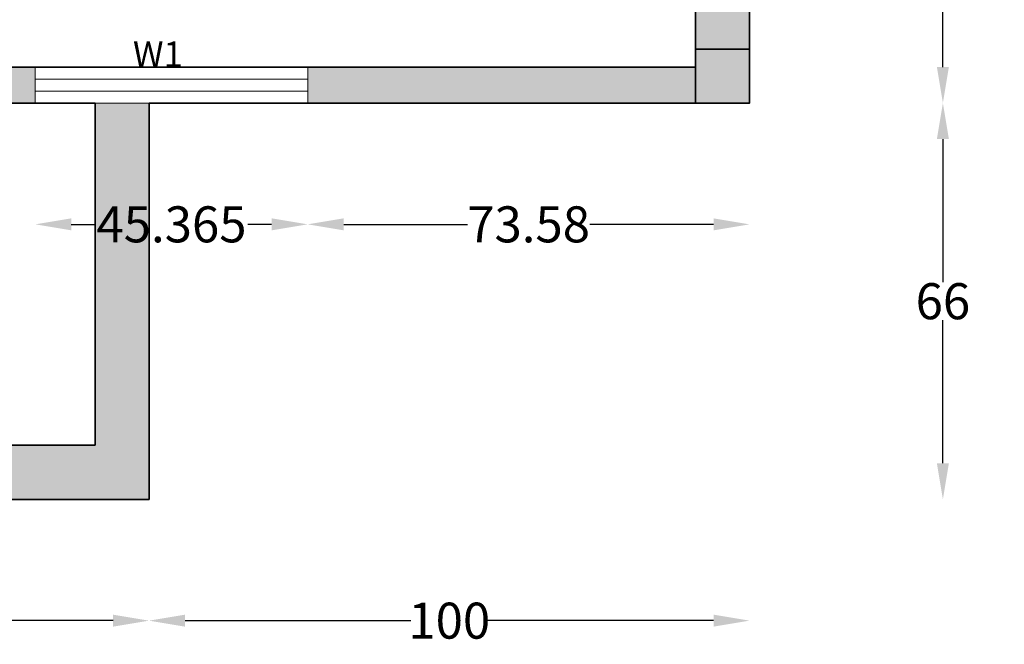
# Model space of a CAD drawing. Units: inches. Extents: x 1994 to 3075, y 3517 to 3950.
# Tile 54 of 58: x 2912 to 3075, y 3517 to 3621. Entities that reach past the tile are written whole.
import ezdxf

# ---------------------------------------------------------------- set-up
doc = ezdxf.new("R2010")
doc.units = ezdxf.units.IN
for name, color, linetype, lineweight in [('A-ANNO-DIMS', 2, 'Continuous', 18), ('A-ANNO-TEXT', 7, 'Continuous', 18), ('A-COLS', 7, 'Continuous', 35), ('A-COLS-PATT', 6, 'Continuous', 13), ('A-GLAZ', 4, 'Continuous', 18), ('A-WALL', 7, 'Continuous', 35), ('A-WALL-PATT', 252, 'Continuous', 13)]:
    doc.layers.add(name, color=color, linetype=linetype, lineweight=lineweight)
doc.styles.get("Standard").update_dxf_attribs({"font": 'arial.ttf'})
doc.dimstyles.get("Standard").update_dxf_attribs({"dimtxt": 6, "dimasz": 6, "dimexe": 0.18, "dimexo": 0.0625, "dimgap": 0.09, "dimtad": 0, "dimtih": 1, "dimtoh": 1, "dimdec": 4, "dimzin": 0, "dimdsep": 46, "dimlunit": 4, "dimtxsty": 'Standard', "dimcen": 0.09, "dimse1": 1, "dimse2": 1, "dimadec": 0, "dimazin": 0, "dimtfac": 1, "dimtdec": 4, "dimtofl": 0, "dimtmove": 0, "dimatfit": 3, "dimfxl": 1, "dimtolj": 1, "dimtzin": 0, "dimarcsym": 0})

# ---------------------------------------------------------------- blocks, each defined once
blk = doc.blocks.new('*D34')
at = {"layer": 'A-ANNO-DIMS', "color": 0, "lineweight": -2, "transparency": 16777216}
for p, q in [((2816.07, 3520.93), (2865.14, 3520.93)), ((2927.07, 3520.93), (2878.01, 3520.93))]:
    blk.add_line(p, q, dxfattribs=at)
at = {"layer": 'A-ANNO-DIMS', "color": 0, "transparency": 16777216}
for points in [[(2816.07, 3521.93), (2816.07, 3519.93), (2810.07, 3520.93)], [(2927.07, 3521.93), (2927.07, 3519.93), (2933.07, 3520.93)]]:
    blk.add_solid(points, dxfattribs=at)
at = {"layer": 'Defpoints', "color": 0, "transparency": 16777216}
for p in [(2810.07, 3541.13), (2933.07, 3541.13), (2933.07, 3520.93)]:
    blk.add_point(p, dxfattribs=at)
at = {"layer": 'A-ANNO-DIMS', "color": 0, "transparency": 16777216, "insert": (2871.57, 3520.93), "char_height": 6, "attachment_point": 5}
blk.add_mtext('\\A1;123', dxfattribs=at)
blk = doc.blocks.new('*D35')
at = {"layer": 'A-ANNO-DIMS', "color": 0, "lineweight": -2, "transparency": 16777216}
for p, q in [((2939.07, 3520.93), (2976.65, 3520.93)), ((3027.07, 3520.93), (2989.5, 3520.93))]:
    blk.add_line(p, q, dxfattribs=at)
at = {"layer": 'A-ANNO-DIMS', "color": 0, "transparency": 16777216}
for points in [[(2939.07, 3521.93), (2939.07, 3519.93), (2933.07, 3520.93)], [(3027.07, 3521.93), (3027.07, 3519.93), (3033.07, 3520.93)]]:
    blk.add_solid(points, dxfattribs=at)
at = {"layer": 'Defpoints', "color": 0, "transparency": 16777216}
for p in [(3033.07, 3607.13), (2933.07, 3541.13), (3033.07, 3520.93)]:
    blk.add_point(p, dxfattribs=at)
at = {"layer": 'A-ANNO-DIMS', "color": 0, "transparency": 16777216, "insert": (2983.07, 3520.93), "char_height": 6, "attachment_point": 5}
blk.add_mtext('\\A1;100', dxfattribs=at)
blk = doc.blocks.new('*D36')
at = {"layer": 'A-ANNO-DIMS', "color": 0, "lineweight": -2, "transparency": 16777216}
for p, q in [((3065.27, 3601.13), (3065.27, 3577.28)), ((3065.27, 3547.13), (3065.27, 3570.97))]:
    blk.add_line(p, q, dxfattribs=at)
at = {"layer": 'A-ANNO-DIMS', "color": 0, "transparency": 16777216}
for points in [[(3064.27, 3601.13), (3066.27, 3601.13), (3065.27, 3607.13)], [(3064.27, 3547.13), (3066.27, 3547.13), (3065.27, 3541.13)]]:
    blk.add_solid(points, dxfattribs=at)
at = {"layer": 'Defpoints', "color": 0, "transparency": 16777216}
for p in [(3033.07, 3607.13), (3065.27, 3607.13), (2933.07, 3541.13)]:
    blk.add_point(p, dxfattribs=at)
at = {"layer": 'A-ANNO-DIMS', "color": 0, "transparency": 16777216, "insert": (3065.27, 3574.13), "char_height": 6, "attachment_point": 5}
blk.add_mtext('\\A1;66', dxfattribs=at)
blk = doc.blocks.new('*D37')
at = {"layer": 'A-ANNO-DIMS', "color": 0, "lineweight": -2, "transparency": 16777216}
for p, q in [((3065.27, 3670.11), (3065.27, 3644.77)), ((3065.27, 3613.13), (3065.27, 3638.47))]:
    blk.add_line(p, q, dxfattribs=at)
at = {"layer": 'A-ANNO-DIMS', "color": 0, "transparency": 16777216}
for points in [[(3064.27, 3670.11), (3066.27, 3670.11), (3065.27, 3676.11)], [(3064.27, 3613.13), (3066.27, 3613.13), (3065.27, 3607.13)]]:
    blk.add_solid(points, dxfattribs=at)
at = {"layer": 'Defpoints', "color": 0, "transparency": 16777216}
for p in [(3033.07, 3676.11), (3065.27, 3676.11), (3033.07, 3607.13)]:
    blk.add_point(p, dxfattribs=at)
at = {"layer": 'A-ANNO-DIMS', "color": 0, "transparency": 16777216, "insert": (3065.27, 3641.62), "char_height": 6, "attachment_point": 5}
blk.add_mtext('\\A1;68.99', dxfattribs=at)
blk = doc.blocks.new('*D47')
at = {"layer": 'A-ANNO-DIMS', "color": 0, "lineweight": -2, "transparency": 16777216}
for p, q in [((2920.13, 3586.93), (2924.12, 3586.93)), ((2953.49, 3586.93), (2949.5, 3586.93))]:
    blk.add_line(p, q, dxfattribs=at)
at = {"layer": 'A-ANNO-DIMS', "color": 0, "transparency": 16777216}
for points in [[(2920.13, 3587.93), (2920.13, 3585.93), (2914.13, 3586.93)], [(2953.49, 3587.93), (2953.49, 3585.93), (2959.49, 3586.93)]]:
    blk.add_solid(points, dxfattribs=at)
at = {"layer": 'Defpoints', "color": 0, "transparency": 16777216}
for p in [(2914.13, 3607.13), (2959.49, 3607.13), (2914.13, 3586.93)]:
    blk.add_point(p, dxfattribs=at)
at = {"layer": 'A-ANNO-DIMS', "color": 0, "transparency": 16777216, "insert": (2936.81, 3586.93), "char_height": 6, "attachment_point": 5}
blk.add_mtext('\\A1;45.365', dxfattribs=at)
blk = doc.blocks.new('*D48')
at = {"layer": 'A-ANNO-DIMS', "color": 0, "lineweight": -2, "transparency": 16777216}
for p, q in [((2965.49, 3586.93), (2986.09, 3586.93)), ((3027.07, 3586.93), (3006.48, 3586.93))]:
    blk.add_line(p, q, dxfattribs=at)
at = {"layer": 'A-ANNO-DIMS', "color": 0, "transparency": 16777216}
for points in [[(2965.49, 3587.93), (2965.49, 3585.93), (2959.49, 3586.93)], [(3027.07, 3587.93), (3027.07, 3585.93), (3033.07, 3586.93)]]:
    blk.add_solid(points, dxfattribs=at)
at = {"layer": 'Defpoints', "color": 0, "transparency": 16777216}
for p in [(2959.49, 3607.13), (3033.07, 3607.13), (2959.49, 3586.93)]:
    blk.add_point(p, dxfattribs=at)
at = {"layer": 'A-ANNO-DIMS', "color": 0, "transparency": 16777216, "insert": (2996.28, 3586.93), "char_height": 6, "attachment_point": 5}
blk.add_mtext('\\A1;73.58', dxfattribs=at)

msp = doc.modelspace()

# ---------------------------------------------------------------- hatches: boundary and pattern name
at = {"layer": 'A-COLS-PATT'}
h = msp.add_hatch(color=256, dxfattribs=at)
h.dxf.hatch_style = 1
h.paths.add_polyline_path([(2678.072, 3914.1269), (2669.072, 3914.1269), (2669.072, 3905.1269), (2678.072, 3905.1269)])
h.paths.add_polyline_path([(2816.072, 3914.1269), (2807.072, 3914.1269), (2807.072, 3905.1269), (2816.072, 3905.1269)])
h.paths.add_polyline_path([(2894.9096, 3914.1269), (2885.9096, 3914.1269), (2885.9096, 3905.1269), (2894.9096, 3905.1269)])
h.paths.add_polyline_path([(3033.072, 3914.1269), (3024.072, 3914.1269), (3024.072, 3905.1269), (3033.072, 3905.1269)])
h.paths.add_polyline_path([(3033.072, 3764.1269), (3024.072, 3764.1269), (3024.072, 3755.1269), (3033.072, 3755.1269)])
h.paths.add_polyline_path([(2895.072, 3764.1269), (2886.072, 3764.1269), (2886.072, 3755.1269), (2895.072, 3755.1269)])
h.paths.add_polyline_path([(2816.072, 3764.1269), (2807.072, 3764.1269), (2807.072, 3755.1269), (2816.072, 3755.1269)])
h.paths.add_polyline_path([(2678.072, 3764.1269), (2669.072, 3764.1269), (2669.072, 3755.1269), (2678.072, 3755.1269)])
h.paths.add_polyline_path([(2678.072, 3664.1269), (2669.072, 3664.1269), (2669.072, 3655.1269), (2678.072, 3655.1269)])
h.paths.add_polyline_path([(2816.072, 3664.1269), (2807.072, 3664.1269), (2807.072, 3655.1269), (2816.072, 3655.1269)])
h.paths.add_polyline_path([(3033.072, 3616.1269), (3024.072, 3616.1269), (3024.072, 3607.1269), (3033.072, 3607.1269)])
h.paths.add_polyline_path([(2894.9096, 3616.1269), (2885.9096, 3616.1269), (2885.9096, 3607.1269), (2894.9096, 3607.1269)])
h.paths.add_polyline_path([(2816.072, 3559.1269), (2807.072, 3559.1269), (2807.072, 3550.1269), (2816.072, 3550.1269)])
h.paths.add_polyline_path([(2678.072, 3559.1269), (2669.072, 3559.1269), (2669.072, 3550.1269), (2678.072, 3550.1269)])
at = {"layer": 'A-WALL-PATT'}
h = msp.add_hatch(color=256, dxfattribs=at)
h.dxf.hatch_style = 1
h.paths.add_polyline_path([(2678.072, 3755.1269), (2669.072, 3755.1269), (2669.072, 3718.5523), (2678.072, 3718.5523)])
h.paths.add_polyline_path([(2807.072, 3761.1269), (2678.072, 3761.1269), (2678.072, 3755.1269), (2807.072, 3755.1269)])
h.paths.add_polyline_path([(2678.072, 3812.7371), (2669.072, 3812.7371), (2669.072, 3809.7371), (2669.072, 3764.1269), (2678.072, 3764.1269)])
h.paths.add_polyline_path([(2678.072, 3905.1269), (2669.072, 3905.1269), (2669.072, 3868.7491), (2678.072, 3868.7491)])
h.paths.add_polyline_path([(2723.826, 3914.1269), (2720.826, 3914.1269), (2678.072, 3914.1269), (2678.072, 3905.1269), (2723.826, 3905.1269)])
h.paths.add_polyline_path([(2807.072, 3914.1269), (2779.838, 3914.1269), (2779.838, 3905.1269), (2807.072, 3905.1269)])
h.paths.add_polyline_path([(2837.6979, 3914.1269), (2834.6979, 3914.1269), (2820.9062, 3914.1269), (2816.072, 3914.1269), (2816.072, 3905.1269), (2837.6979, 3905.1269)])
h.paths.add_polyline_path([(2885.9096, 3914.1269), (2869.71, 3914.1269), (2869.71, 3905.1269), (2876.9183, 3905.1269), (2885.9096, 3905.1269)])
h.paths.add_polyline_path([(2933.6904, 3914.1269), (2930.6904, 3914.1269), (2894.9096, 3914.1269), (2894.9096, 3905.1269), (2933.6904, 3905.1269)])
h.paths.add_polyline_path([(3024.072, 3914.1269), (2989.7025, 3914.1269), (2989.7025, 3905.1269), (3024.072, 3905.1269)])
h.paths.add_polyline_path([(3033.072, 3905.1269), (3024.072, 3905.1269), (3024.072, 3861.4192), (3033.072, 3861.4192)])
h.paths.add_polyline_path([(3033.072, 3805.4072), (3024.072, 3805.4072), (3024.072, 3764.1269), (3033.072, 3764.1269)])
h.paths.add_polyline_path([(3033.072, 3755.1269), (3024.072, 3755.1269), (3024.072, 3732.1247), (3033.072, 3732.1247), (3033.072, 3735.1247)])
h.paths.add_polyline_path([(3024.072, 3761.1269), (2895.072, 3761.1269), (2895.072, 3755.1269), (3024.072, 3755.1269)])
h.paths.add_polyline_path([(3033.072, 3676.1126), (3024.072, 3676.1126), (3024.072, 3616.1269), (3033.072, 3616.1269)])
h.paths.add_polyline_path([(3024.072, 3613.1269), (2959.4908, 3613.1269), (2959.4908, 3607.1269), (3024.072, 3607.1269)])
h.paths.add_polyline_path([(2914.1254, 3613.1269), (2894.9096, 3613.1269), (2894.9096, 3607.1269), (2914.1254, 3607.1269)])
h.paths.add_polyline_path([(2885.9096, 3613.1269), (2852.072, 3613.1269), (2852.072, 3607.1269), (2885.9096, 3607.1269)])
h.paths.add_polyline_path([(2822.072, 3613.1269), (2810.072, 3613.1269), (2810.072, 3559.1269), (2816.072, 3559.1269), (2816.072, 3607.1269), (2822.072, 3607.1269)])
h.paths.add_polyline_path([(2933.072, 3607.1269), (2924.072, 3607.1269), (2924.072, 3550.1269), (2892.072, 3550.1269), (2816.072, 3550.1269), (2810.072, 3550.1269), (2810.072, 3541.1269), (2892.072, 3541.1269), (2933.072, 3541.1269)])
h.paths.add_polyline_path([(2807.072, 3559.1269), (2678.072, 3559.1269), (2678.072, 3550.1269), (2807.072, 3550.1269)])
h.paths.add_polyline_path([(2678.072, 3655.1269), (2669.072, 3655.1269), (2669.072, 3559.1269), (2678.072, 3559.1269)])
h.paths.add_polyline_path([(2678.072, 3686.5403), (2669.072, 3686.5403), (2669.072, 3664.1269), (2678.072, 3664.1269)])
h.paths.add_polyline_path([(2807.072, 3661.1269), (2678.072, 3661.1269), (2678.072, 3655.1269), (2807.072, 3655.1269)])
h.paths.add_polyline_path([(2816.072, 3755.1269), (2810.072, 3755.1269), (2810.072, 3703.1269), (2816.072, 3703.1269)])
h.paths.add_polyline_path([(2816.072, 3905.1269), (2810.072, 3905.1269), (2810.072, 3803.1269), (2816.072, 3803.1269), (2816.072, 3815.1269)])
h.paths.add_polyline_path([(2886.072, 3821.1269), (2852.072, 3821.1269), (2852.072, 3815.1269), (2886.072, 3815.1269)])
h.paths.add_polyline_path([(2822.072, 3821.1269), (2816.072, 3821.1269), (2816.072, 3815.1269), (2822.072, 3815.1269)])
h.paths.add_polyline_path([(2892.072, 3905.1269), (2886.072, 3905.1269), (2886.072, 3803.1269), (2892.072, 3803.1269)])

# ---------------------------------------------------------------- linework, layer by layer
at = {"layer": 'A-COLS'}
msp.add_lwpolyline([(3024.072, 3607.1269), (3033.072, 3607.1269), (3033.072, 3616.1269), (3024.072, 3616.1269)], close=True, dxfattribs=at)
at = {"layer": 'A-GLAZ'}
for p, q in [((2914.1254, 3607.1269), (2914.1254, 3613.1269)), ((2914.1254, 3613.1269), (2959.4908, 3613.1269)), ((2959.4908, 3613.1269), (2959.4908, 3607.1269)), ((2914.1254, 3611.1269), (2959.4908, 3611.1269)), ((2914.1254, 3609.1269), (2959.4908, 3609.1269)), ((2959.4908, 3607.1269), (2914.1254, 3607.1269))]:
    msp.add_line(p, q, dxfattribs=at)
at = {"layer": 'A-WALL'}
for p, q in [((3033.072, 3914.1269), (3033.072, 3607.1269)), ((3024.072, 3905.1269), (3024.072, 3607.1269)), ((2894.9096, 3613.1269), (3024.072, 3613.1269)), ((2892.072, 3607.1269), (2924.072, 3607.1269)), ((2924.072, 3607.1269), (2924.072, 3550.1269)), ((2933.072, 3607.1269), (2933.072, 3541.1269)), ((2933.072, 3607.1269), (3024.072, 3607.1269)), ((3024.072, 3607.1269), (3033.072, 3607.1269)), ((2892.072, 3550.1269), (2924.072, 3550.1269)), ((2892.072, 3541.1269), (2933.072, 3541.1269))]:
    msp.add_line(p, q, dxfattribs=at)

# ---------------------------------------------------------------- texts
at = {"layer": 'A-ANNO-TEXT', "insert": (2930.3939, 3617.3895), "char_height": 4.24528, "attachment_point": 1}
msp.add_mtext_dynamic_manual_height_columns('W1', width=102.693633, gutter_width=21.2264, heights=[0], dxfattribs=at)

# ---------------------------------------------------------------- dimensions: what is measured, and where the dimension line sits
at = {"layer": 'A-ANNO-DIMS'}
for base, p1, p2, angle, override, picture, middle in [((3065.272, 3676.1126), (3033.072, 3607.1269), (3033.072, 3676.1126), 90, {"dimdec": 2, "dimlfac": 1, "dimrnd": 0, "dimzin": 0, "dimdsep": 46, "dimlunit": 2}, '*D37', (3065.272, 3641.6197)), ((2914.1254, 3586.9269), (2959.4908, 3607.1269), (2914.1254, 3607.1269), 180, {"dimdec": 3, "dimlfac": 1, "dimrnd": 0, "dimzin": 0, "dimdsep": 46, "dimlunit": 2}, '*D47', (2936.8081, 3586.9269)), ((3065.272, 3607.1269), (2933.072, 3541.1269), (3033.072, 3607.1269), 90, {"dimdec": 0, "dimlfac": 1, "dimrnd": 0, "dimzin": 0, "dimdsep": 46, "dimlunit": 2}, '*D36', (3065.272, 3574.1269)), ((2959.4908, 3586.9269), (3033.072, 3607.1269), (2959.4908, 3607.1269), 180, {"dimdec": 2, "dimlfac": 1, "dimrnd": 0, "dimzin": 0, "dimdsep": 46, "dimlunit": 2}, '*D48', (2996.2814, 3586.9269))]:
    dim = msp.add_linear_dim(base=base, p1=p1, p2=p2, angle=angle, dimstyle='Standard', override=override, dxfattribs=at)
    dim.commit()
    dim.dimension.update_dxf_attribs({"geometry": picture, "text_midpoint": middle})
for base, p1, p2, picture, middle in [((3033.072, 3520.9269), (2933.072, 3541.1269), (3033.072, 3607.1269), '*D35', (2983.072, 3520.9269)), ((2933.072, 3520.9269), (2810.072, 3541.1269), (2933.072, 3541.1269), '*D34', (2871.572, 3520.9269))]:
    dim = msp.add_linear_dim(base=base, p1=p1, p2=p2, dimstyle='Standard', override={"dimdec": 0, "dimlfac": 1, "dimrnd": 0, "dimzin": 0, "dimdsep": 46, "dimlunit": 2}, dxfattribs=at)
    dim.commit()
    dim.dimension.update_dxf_attribs({"geometry": picture, "text_midpoint": middle})

doc.saveas('drawing.dxf')
